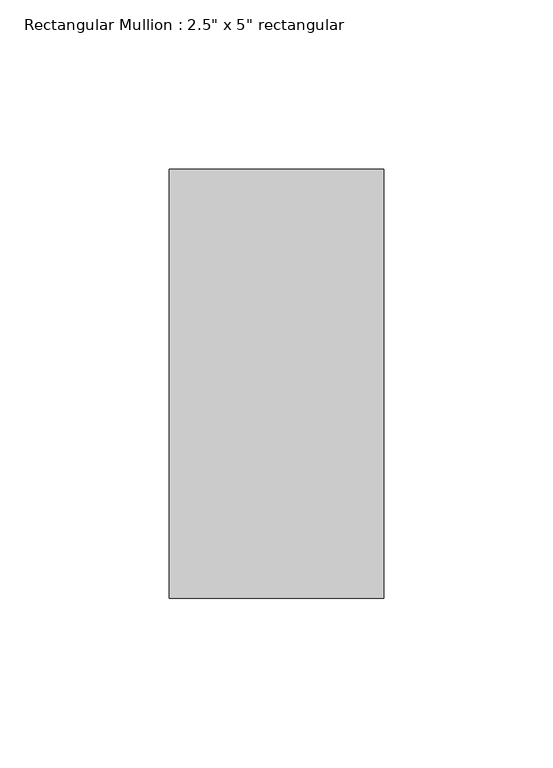
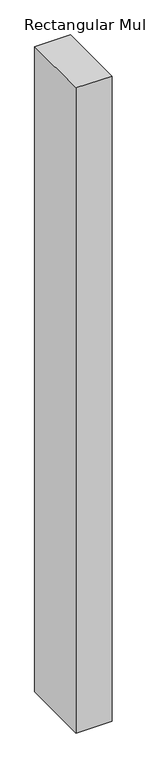
"""IFC4 building model written with IfcOpenShell, lengths in millimetres: member geometry."""

from ifc_helpers import new_model, si_unit, frame, origin, place, context, project, spatial, polyline, outline, extrude, source, transform, mapped, element, save


def member_74da8ab1(model_context):
    return source(origin(), model_context, "Body", "SweptSolid", [
        extrude(outline(polyline([(0.0, 63.5), (0.0, -63.5), (-63.5, -63.5), (-63.5, 63.5), (0.0, 63.5)])), frame((0.0, 0.0, -1208.6166667), z_axis=(0.0, 0.0, 1.0), x_axis=(1.0, 0.0, 0.0)), (0.0, 0.0, 1.0), 1208.6166667),
    ])


if __name__ == "__main__":
    model = new_model("IFC4")
    model_context = context("Model", 3, world=origin())
    ifc_project = project(units=[si_unit("LENGTHUNIT", "METRE", prefix="MILLI")], contexts=[model_context])
    site = spatial("IfcSite", under=ifc_project)
    building = spatial("IfcBuilding", under=site)
    placement = place(None, origin())
    member_shape = member_74da8ab1(model_context)
    element("IfcMember", 1, ObjectType="Rectangular Mullion : 2.5\" x 5\" rectangular", at=placement, inside=building, context=model_context, shape_type="MappedRepresentation", body=[
        mapped(member_shape, transform((0.0, 0.0, 0.0), x_axis=(1.0, 0.0, 0.0), y_axis=(0.0, 1.0, 0.0), z_axis=(0.0, 0.0, 1.0))),
    ])
    save(model, "model.ifc")

# Revit data of these elements
# Type "Rectangular Mullion : 2.5\" x 5\" rectangular"
#   built-in parameter 1007304 = 0.416667 (stored number, unit not read)
#   built-in parameter 1007301 = 0.104167 (stored number, unit not read)
#   built-in parameter 1007300 = 0.104167 (stored number, unit not read)
# Element 1 (IfcMember, "Rectangular Mullion : 2.5\" x 5\" rectangular")
#   Materials on its faces: "Aluminum"
# Materials
#   "Aluminum": class "Metal", colour RGB 247 247 247, transparency 0, Description = "Aluminum 6061", Cost = 0
